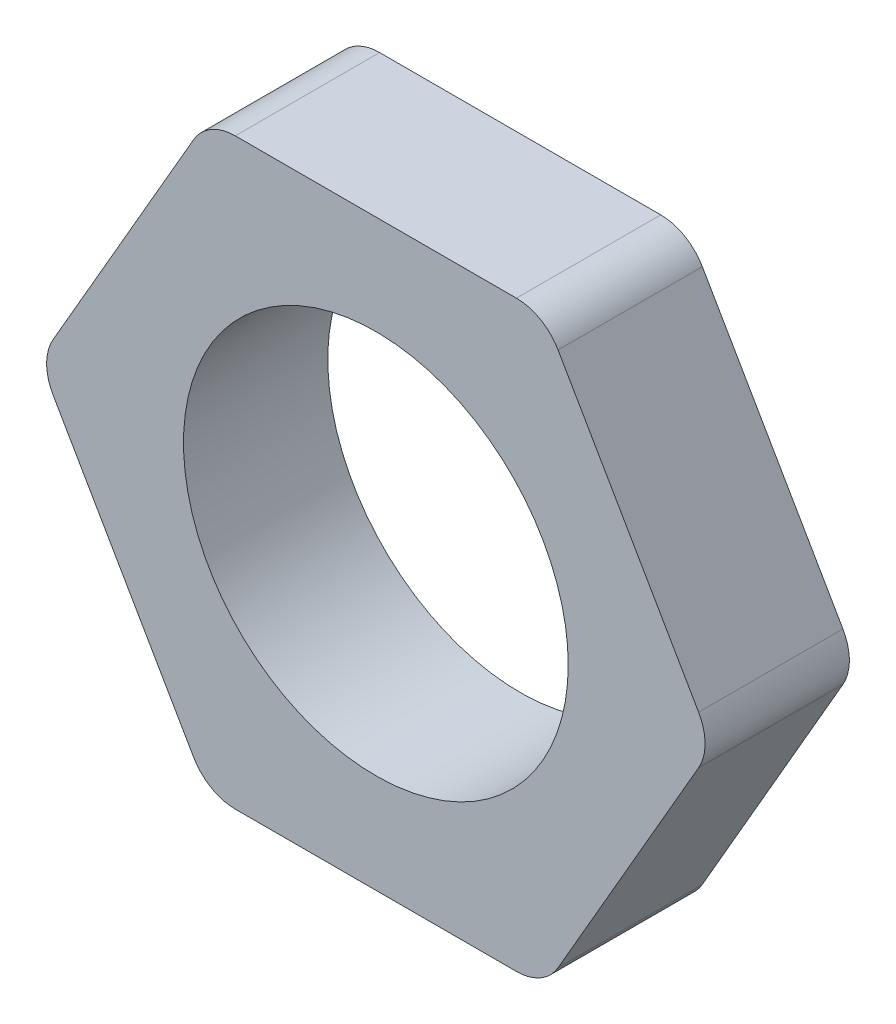
SolidWorks part; units mm, degrees
material "Plain Carbon Steel"
ref_plane "Front Plane" through (0, 0, 0) normal (0, 0, 1) x (1, 0, 0)
ref_plane "Top Plane" through (0, 0, 0) normal (0, 1, 0) x (1, 0, 0)
ref_plane "Right Plane" through (0, 0, 0) normal (1, 0, 0) x (0, 0, -1)
sketch "Hex Profile Sketch" plane through (0, 0, 0) normal (0, 0, 1) x (1, 0, 0)
  line L1 (3.5, -6.0622) -> (7, 0)
  line L2 (7, 0) -> (3.5, 6.0622)
  line L3 (3.5, 6.0622) -> (-3.5, 6.0622)
  line L4 (-3.5, 6.0622) -> (-7, 0)
  line L5 (-7, 0) -> (-3.5, -6.0622)
  line L6 (-3.5, -6.0622) -> (3.5, -6.0622)
  circle A0 centre (0, 0) radius 6.0622 construction
  dimension "D1" = 14
extrude "Hex Body" add sketch "Hex Profile Sketch" along normal blind 3
fillet "Hex Corner Fillets R1" radius 1 6 edges at (7, 0, 1.5) (3.5, -6.0622, 1.5) (-3.5, -6.0622, 1.5) (-7, 0, 1.5) (-3.5, 6.0622, 1.5) (3.5, 6.0622, 1.5)
sketch "Bore Sketch" plane through (0, 0, 3) normal (0, 0, 1) x (1, 0, 0)
  circle A0 centre (0, 0) radius 4
  dimension "D1" = 8
extrude "Bore Ø8" cut sketch "Bore Sketch" against normal blind 3
cosmetic thread "Cosmetic Thread2" parameters "D1"=3, "D2"=9.728
